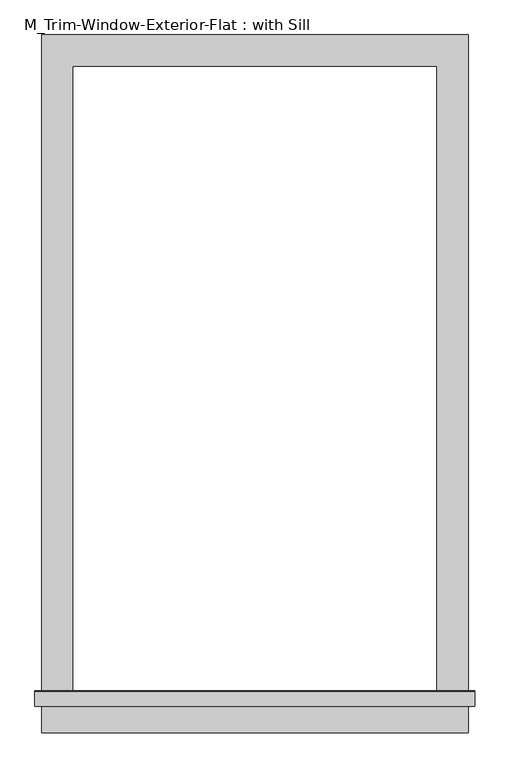
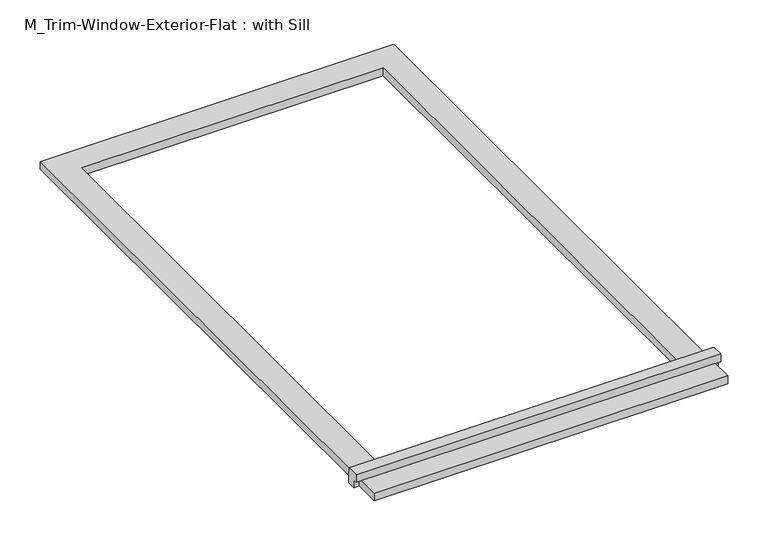
"""IFC4 building model written with IfcOpenShell, lengths in millimetres: proxy geometry, M_Trim-Window-Exterior-Flat : with Sill."""

from ifc_helpers import new_model, si_unit, frame, origin, origin_with_axes, place, context, project, spatial, polyline, outline, extrude, source, transform, mapped, element, save


def m_trim_window_exterior_flat_with_sill_7a42a2ef(model_context):
    return source(origin(), model_context, "Body", "SweptSolid", [
        extrude(outline(polyline([(410.0, -1220.4323709), (410.0, -1280.4323709), (-410.0, -1280.4323709), (-410.0, -1220.4323709), (410.0, -1220.4323709)])), origin_with_axes(), (0.0, 0.0, 1.0), 19.05),
        extrude(outline(polyline([(-1230.0, 38.1), (-1202.4580645, 38.1), (-1200.0, 19.05), (-1200.0, 0.0), (-1220.4323709, 0.0), (-1220.4323709, 19.05), (-1230.0, 19.05), (-1230.0, 38.1)])), frame((-422.7, 0.0, 0.0), z_axis=(1.0, 0.0, 0.0), x_axis=(0.0, 1.0, 0.0)), (0.0, 0.0, 1.0), 845.4),
        extrude(outline(polyline([(-410.0, 60.0), (410.0, 60.0), (410.0, -1200.0), (350.0, -1200.0), (350.0, 0.0), (-350.0, 0.0), (-350.0, -1200.0), (-410.0, -1200.0), (-410.0, 60.0)])), origin_with_axes(), (0.0, 0.0, 1.0), 19.05),
    ])


if __name__ == "__main__":
    model = new_model("IFC4")
    model_context = context("Model", 3, world=origin())
    ifc_project = project(units=[si_unit("LENGTHUNIT", "METRE", prefix="MILLI")], contexts=[model_context])
    site = spatial("IfcSite", under=ifc_project)
    building = spatial("IfcBuilding", under=site)
    placement = place(None, origin())
    m_trim_window_exterior_flat_with_sill_shape = m_trim_window_exterior_flat_with_sill_7a42a2ef(model_context)
    element("IfcBuildingElementProxy", 1, Name="M_Trim-Window-Exterior-Flat : with Sill", ObjectType="M_Trim-Window-Exterior-Flat : with Sill", at=placement, inside=building, context=model_context, shape_type="MappedRepresentation", body=[
        mapped(m_trim_window_exterior_flat_with_sill_shape, transform((0.0, 0.0, 0.0), x_axis=(1.0, 0.0, 0.0), y_axis=(0.0, 1.0, 0.0), z_axis=(0.0, 0.0, 1.0))),
    ])
    save(model, "model.ifc")

# Revit data of these elements
# Type "M_Trim-Window-Exterior-Flat : with Sill"
#   Trim Width = 60 mm
#   Trim Thickness_Picture Frame = 30 mm
#   Trim Thickness_with Sill = 19.05 mm
#   Sill Thickness = 30 mm
#   Opening Width [instance default] = 600 mm
#   Opening Height [instance default] = 900 mm
#   Default Elevation = 1200 mm
#   Sill = yes
#   Picture Frame = no
#   Trim Material [instance default] = none
# Element 1 (IfcBuildingElementProxy, "M_Trim-Window-Exterior-Flat : with Sill")
#   Opening Width = 700 mm
#   Opening Height = 1200 mm
#   Trim Material = Clad - White
#   Materials on its faces: "Clad - White"
# Materials
#   "Clad - White": class "Wood", colour RGB 245 245 243, transparency 0, Cost = 0
